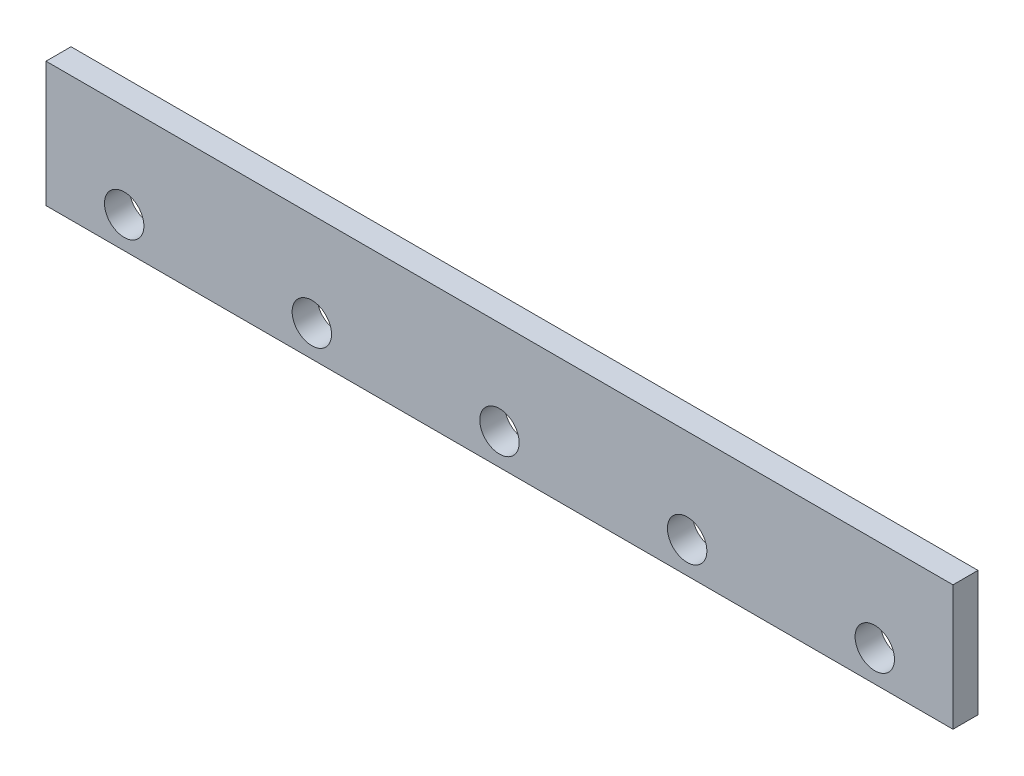
SolidWorks part; units mm, degrees
material "Plain Carbon Steel"
ref_plane "Front Plane" through (0, 0, 0) normal (0, 0, 1) x (1, 0, 0)
ref_plane "Top Plane" through (0, 0, 0) normal (0, 1, 0) x (1, 0, 0)
ref_plane "Right Plane" through (0, 0, 0) normal (1, 0, 0) x (0, 0, -1)
sketch "Bar Profile Sketch" plane through (0, 0, 0) normal (0, 0, 1) x (1, 0, 0)
  line L1 (-290, 40) -> (290, 40)
  line L2 (-290, 40) -> (-290, -40)
  line L3 (-290, -40) -> (290, -40)
  line L4 (290, 40) -> (290, -40)
  line L5 (-290, 40) -> (290, -40) construction
  line L6 (-290, -40) -> (290, 40) construction
  point P0 (0, 0)
  dimension "D1" = 580
  dimension "D2" = 80
extrude "Flat Bar 580x80x16" add sketch "Bar Profile Sketch" along normal blind 16
sketch "Hole Row Sketch" plane through (0, 0, 16) normal (0, 0, 1) x (1, 0, 0)
  line L0 (-290, 40) -> (-290, -40) construction
  line L1 (-290, -40) -> (290, -40) construction
  line L2 (-240, -20) -> (-120, -20) construction
  circle A0 centre (-240, -20) radius 12.6
  circle A1 centre (-120, -20) radius 12.6
  circle A2 centre (0, -20) radius 12.6
  circle A3 centre (120, -20) radius 12.6
  circle A4 centre (240, -20) radius 12.6
  dimension "D1" = 25.2
  dimension "D2" = 50
  dimension "D3" = 20
  dimension "D5" = 120
  dimension "D4" = 5
extrude "Through Holes 5x Pitch 120" cut sketch "Hole Row Sketch" against normal blind 26
